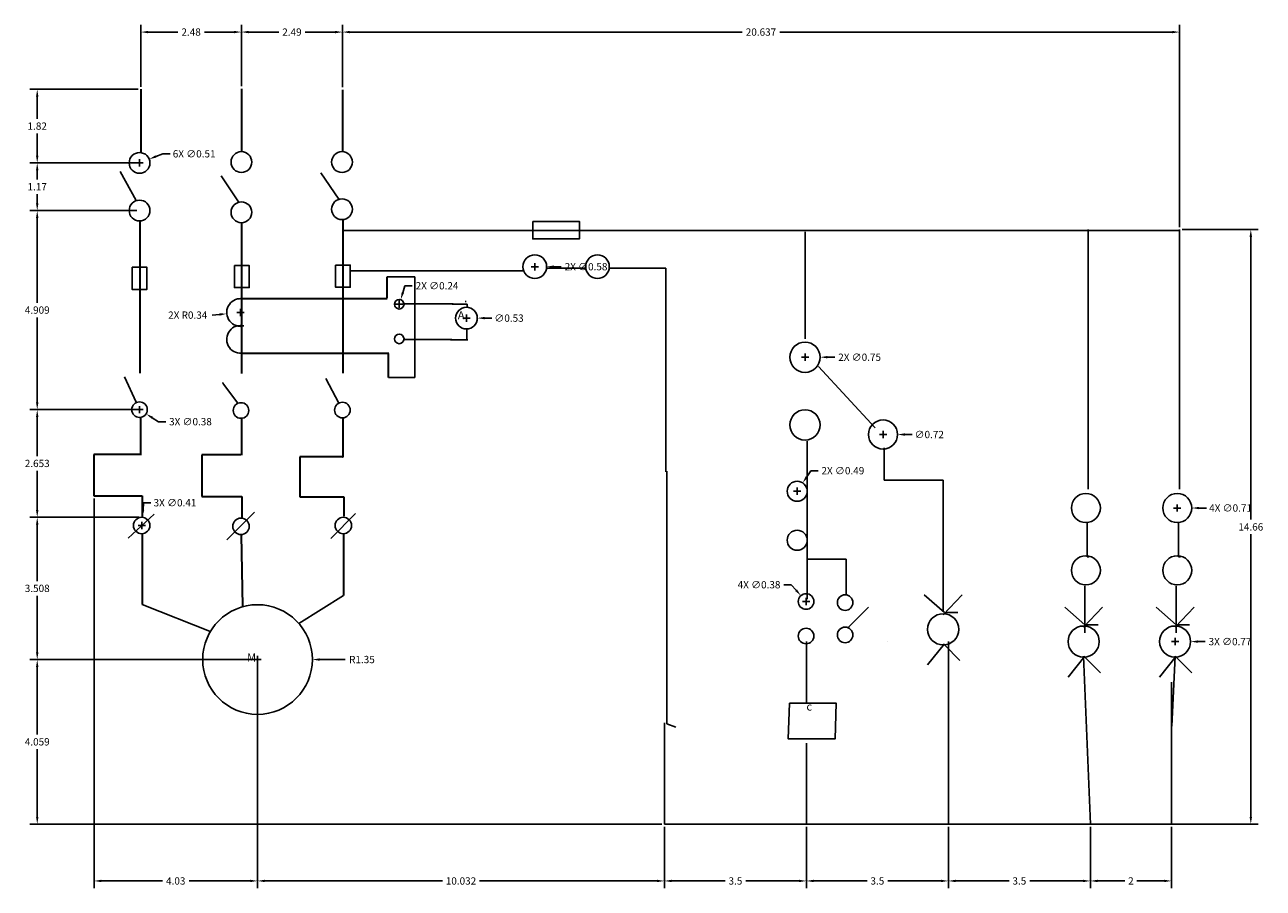
# Model space of a CAD drawing. Units: millimetres. Extents: x 17.2 to 47.7, y -5.7 to 15.6.
import ezdxf

# ---------------------------------------------------------------- set-up
doc = ezdxf.new("R2010")
doc.units = ezdxf.units.MM
doc.header["$MEASUREMENT"] = 0
for name, color, linetype, lineweight in [('A-ANNO-DIMS', 2, 'Continuous', 18), ('E-ANNO-TEXT', 7, 'Continuous', 18), ('E-CTRL-WIRE', 5, 'Continuous', 25), ('E-DEVC-SYMB', 3, 'Continuous', 25), ('E-POWR-WIRE', 1, 'Continuous', 35)]:
    doc.layers.add(name, color=color, linetype=linetype, lineweight=lineweight)
doc.styles.get("Standard").update_dxf_attribs({"font": 'arial.ttf'})
doc.dimstyles.get("Standard").update_dxf_attribs({"dimtxt": 0.18, "dimasz": 0.18, "dimexe": 0.18, "dimexo": 0.0625, "dimgap": 0.09, "dimtad": 0, "dimtih": 1, "dimtoh": 1, "dimdec": 4, "dimzin": 0, "dimdsep": 46, "dimtxsty": 'Standard', "dimcen": 0.09, "dimadec": 0, "dimazin": 0, "dimtfac": 1, "dimtdec": 4, "dimtofl": 0, "dimtmove": 0, "dimatfit": 3, "dimfxl": 1, "dimtolj": 1, "dimtzin": 0, "dimarcsym": 0})

# ---------------------------------------------------------------- blocks, each defined once
blk = doc.blocks.new('*D2')
at = {"layer": 'A-ANNO-DIMS', "color": 0, "lineweight": -2, "transparency": 16777216}
for p, q in [((20.016, 14.072), (20.016, 15.6)), ((22.496, 14.082), (22.496, 15.6)), ((20.196, 15.42), (20.931, 15.42)), ((22.316, 15.42), (21.582, 15.42))]:
    blk.add_line(p, q, dxfattribs=at)
at = {"layer": 'A-ANNO-DIMS', "color": 0, "transparency": 16777216}
for points in [[(20.196, 15.45), (20.196, 15.39), (20.016, 15.42)], [(22.316, 15.45), (22.316, 15.39), (22.496, 15.42)]]:
    blk.add_solid(points, dxfattribs=at)
at = {"layer": 'Defpoints', "color": 0, "transparency": 16777216}
for p in [(22.496, 15.42), (20.016, 14.009), (22.496, 14.02)]:
    blk.add_point(p, dxfattribs=at)
at = {"layer": 'A-ANNO-DIMS', "color": 0, "transparency": 16777216, "insert": (21.256, 15.42), "char_height": 0.18, "attachment_point": 5}
blk.add_mtext('\\A1;2.48', dxfattribs=at)
blk = doc.blocks.new('*D3')
at = {"layer": 'A-ANNO-DIMS', "color": 0, "lineweight": -2, "transparency": 16777216}
for p, q in [((22.496, 14.082), (22.496, 15.6)), ((24.987, 14.061), (24.987, 15.6)), ((22.676, 15.42), (23.416, 15.42)), ((24.807, 15.42), (24.067, 15.42))]:
    blk.add_line(p, q, dxfattribs=at)
at = {"layer": 'A-ANNO-DIMS', "color": 0, "transparency": 16777216}
for points in [[(22.676, 15.45), (22.676, 15.39), (22.496, 15.42)], [(24.807, 15.45), (24.807, 15.39), (24.987, 15.42)]]:
    blk.add_solid(points, dxfattribs=at)
at = {"layer": 'Defpoints', "color": 0, "transparency": 16777216}
for p in [(24.987, 15.42), (22.496, 14.02), (24.987, 13.999)]:
    blk.add_point(p, dxfattribs=at)
at = {"layer": 'A-ANNO-DIMS', "color": 0, "transparency": 16777216, "insert": (23.741, 15.42), "char_height": 0.18, "attachment_point": 5}
blk.add_mtext('\\A1;2.49', dxfattribs=at)
blk = doc.blocks.new('*D4')
at = {"layer": 'A-ANNO-DIMS', "color": 0, "lineweight": -2, "transparency": 16777216}
for p, q in [((24.987, 14.061), (24.987, 15.6)), ((45.623, 10.611), (45.623, 15.6)), ((25.167, 15.42), (34.84, 15.42)), ((45.443, 15.42), (35.77, 15.42))]:
    blk.add_line(p, q, dxfattribs=at)
at = {"layer": 'A-ANNO-DIMS', "color": 0, "transparency": 16777216}
for points in [[(25.167, 15.45), (25.167, 15.39), (24.987, 15.42)], [(45.443, 15.45), (45.443, 15.39), (45.623, 15.42)]]:
    blk.add_solid(points, dxfattribs=at)
at = {"layer": 'Defpoints', "color": 0, "transparency": 16777216}
for p in [(45.623, 15.42), (24.987, 13.999), (45.623, 10.549)]:
    blk.add_point(p, dxfattribs=at)
at = {"layer": 'A-ANNO-DIMS', "color": 0, "transparency": 16777216, "insert": (35.305, 15.42), "char_height": 0.18, "attachment_point": 5}
blk.add_mtext('\\A1;20.637', dxfattribs=at)
blk = doc.blocks.new('*D5')
at = {"layer": 'A-ANNO-DIMS', "color": 0, "lineweight": -2, "transparency": 16777216}
for p, q in [((18.862, 3.921), (18.862, -5.69)), ((22.893, -0.113), (22.893, -5.69)), ((19.042, -5.51), (20.55, -5.51)), ((22.713, -5.51), (21.205, -5.51))]:
    blk.add_line(p, q, dxfattribs=at)
at = {"layer": 'A-ANNO-DIMS', "color": 0, "transparency": 16777216}
for points in [[(19.042, -5.48), (19.042, -5.54), (18.862, -5.51)], [(22.713, -5.48), (22.713, -5.54), (22.893, -5.51)]]:
    blk.add_solid(points, dxfattribs=at)
at = {"layer": 'Defpoints', "color": 0, "transparency": 16777216}
for p in [(18.862, 3.983), (22.893, -0.051), (22.893, -5.51)]:
    blk.add_point(p, dxfattribs=at)
at = {"layer": 'A-ANNO-DIMS', "color": 0, "transparency": 16777216, "insert": (20.877, -5.51), "char_height": 0.18, "attachment_point": 5}
blk.add_mtext('\\A1;4.03', dxfattribs=at)
blk = doc.blocks.new('*D6')
at = {"layer": 'A-ANNO-DIMS', "color": 0, "lineweight": -2, "transparency": 16777216}
for p, q in [((22.893, -0.113), (22.893, -5.69)), ((32.925, -4.172), (32.925, -5.69)), ((23.073, -5.51), (27.455, -5.51)), ((32.745, -5.51), (28.364, -5.51))]:
    blk.add_line(p, q, dxfattribs=at)
at = {"layer": 'A-ANNO-DIMS', "color": 0, "transparency": 16777216}
for points in [[(23.073, -5.48), (23.073, -5.54), (22.893, -5.51)], [(32.745, -5.48), (32.745, -5.54), (32.925, -5.51)]]:
    blk.add_solid(points, dxfattribs=at)
at = {"layer": 'Defpoints', "color": 0, "transparency": 16777216}
for p in [(22.893, -0.051), (32.925, -4.11), (32.925, -5.51)]:
    blk.add_point(p, dxfattribs=at)
at = {"layer": 'A-ANNO-DIMS', "color": 0, "transparency": 16777216, "insert": (27.909, -5.51), "char_height": 0.18, "attachment_point": 5}
blk.add_mtext('\\A1;10.032', dxfattribs=at)
blk = doc.blocks.new('*D7')
at = {"layer": 'A-ANNO-DIMS', "color": 0, "lineweight": -2, "transparency": 16777216}
for p, q in [((32.925, -4.172), (32.925, -5.69)), ((36.425, -4.172), (36.425, -5.69)), ((33.105, -5.51), (34.421, -5.51)), ((36.245, -5.51), (34.93, -5.51))]:
    blk.add_line(p, q, dxfattribs=at)
at = {"layer": 'A-ANNO-DIMS', "color": 0, "transparency": 16777216}
for points in [[(33.105, -5.48), (33.105, -5.54), (32.925, -5.51)], [(36.245, -5.48), (36.245, -5.54), (36.425, -5.51)]]:
    blk.add_solid(points, dxfattribs=at)
at = {"layer": 'Defpoints', "color": 0, "transparency": 16777216}
for p in [(32.925, -4.11), (36.425, -4.11), (36.425, -5.51)]:
    blk.add_point(p, dxfattribs=at)
at = {"layer": 'A-ANNO-DIMS', "color": 0, "transparency": 16777216, "insert": (34.675, -5.51), "char_height": 0.18, "attachment_point": 5}
blk.add_mtext('\\A1;3.5', dxfattribs=at)
blk = doc.blocks.new('*D8')
at = {"layer": 'A-ANNO-DIMS', "color": 0, "lineweight": -2, "transparency": 16777216}
for p, q in [((36.425, -4.172), (36.425, -5.69)), ((39.925, -4.172), (39.925, -5.69)), ((36.605, -5.51), (37.921, -5.51)), ((39.745, -5.51), (38.43, -5.51))]:
    blk.add_line(p, q, dxfattribs=at)
at = {"layer": 'A-ANNO-DIMS', "color": 0, "transparency": 16777216}
for points in [[(36.605, -5.48), (36.605, -5.54), (36.425, -5.51)], [(39.745, -5.48), (39.745, -5.54), (39.925, -5.51)]]:
    blk.add_solid(points, dxfattribs=at)
at = {"layer": 'Defpoints', "color": 0, "transparency": 16777216}
for p in [(36.425, -4.11), (39.925, -4.11), (39.925, -5.51)]:
    blk.add_point(p, dxfattribs=at)
at = {"layer": 'A-ANNO-DIMS', "color": 0, "transparency": 16777216, "insert": (38.175, -5.51), "char_height": 0.18, "attachment_point": 5}
blk.add_mtext('\\A1;3.5', dxfattribs=at)
blk = doc.blocks.new('*D9')
at = {"layer": 'A-ANNO-DIMS', "color": 0, "lineweight": -2, "transparency": 16777216}
for p, q in [((39.925, -4.172), (39.925, -5.69)), ((43.425, -4.172), (43.425, -5.69)), ((40.105, -5.51), (41.421, -5.51)), ((43.245, -5.51), (41.93, -5.51))]:
    blk.add_line(p, q, dxfattribs=at)
at = {"layer": 'A-ANNO-DIMS', "color": 0, "transparency": 16777216}
for points in [[(40.105, -5.48), (40.105, -5.54), (39.925, -5.51)], [(43.245, -5.48), (43.245, -5.54), (43.425, -5.51)]]:
    blk.add_solid(points, dxfattribs=at)
at = {"layer": 'Defpoints', "color": 0, "transparency": 16777216}
for p in [(39.925, -4.11), (43.425, -4.11), (43.425, -5.51)]:
    blk.add_point(p, dxfattribs=at)
at = {"layer": 'A-ANNO-DIMS', "color": 0, "transparency": 16777216, "insert": (41.675, -5.51), "char_height": 0.18, "attachment_point": 5}
blk.add_mtext('\\A1;3.5', dxfattribs=at)
blk = doc.blocks.new('*D10')
at = {"layer": 'A-ANNO-DIMS', "color": 0, "lineweight": -2, "transparency": 16777216}
for p, q in [((43.425, -4.172), (43.425, -5.69)), ((45.425, -4.172), (45.425, -5.69)), ((43.605, -5.51), (44.276, -5.51)), ((45.245, -5.51), (44.575, -5.51))]:
    blk.add_line(p, q, dxfattribs=at)
at = {"layer": 'A-ANNO-DIMS', "color": 0, "transparency": 16777216}
for points in [[(43.605, -5.48), (43.605, -5.54), (43.425, -5.51)], [(45.245, -5.48), (45.245, -5.54), (45.425, -5.51)]]:
    blk.add_solid(points, dxfattribs=at)
at = {"layer": 'Defpoints', "color": 0, "transparency": 16777216}
for p in [(43.425, -4.11), (45.425, -4.11), (45.425, -5.51)]:
    blk.add_point(p, dxfattribs=at)
at = {"layer": 'A-ANNO-DIMS', "color": 0, "transparency": 16777216, "insert": (44.425, -5.51), "char_height": 0.18, "attachment_point": 5}
blk.add_mtext('\\A1;2', dxfattribs=at)
blk = doc.blocks.new('*D11')
at = {"layer": 'A-ANNO-DIMS', "color": 0, "lineweight": -2, "transparency": 16777216}
for p, q in [((45.686, 10.549), (47.561, 10.549)), ((47.381, 10.369), (47.381, 3.401)), ((47.381, -3.93), (47.381, 3.038)), ((45.488, -4.11), (47.561, -4.11))]:
    blk.add_line(p, q, dxfattribs=at)
at = {"layer": 'A-ANNO-DIMS', "color": 0, "transparency": 16777216}
for points in [[(47.351, 10.369), (47.411, 10.369), (47.381, 10.549)], [(47.351, -3.93), (47.411, -3.93), (47.381, -4.11)]]:
    blk.add_solid(points, dxfattribs=at)
at = {"layer": 'Defpoints', "color": 0, "transparency": 16777216}
for p in [(45.623, 10.549), (47.381, 10.549), (45.425, -4.11)]:
    blk.add_point(p, dxfattribs=at)
at = {"layer": 'A-ANNO-DIMS', "color": 0, "transparency": 16777216, "insert": (47.381, 3.219), "char_height": 0.18, "attachment_point": 5}
blk.add_mtext('\\A1;14.66', dxfattribs=at)
blk = doc.blocks.new('*D12')
at = {"layer": 'A-ANNO-DIMS', "color": 0, "lineweight": -2, "transparency": 16777216}
for p, q in [((19.954, 14.009), (17.282, 14.009)), ((17.462, 13.829), (17.462, 13.283)), ((17.462, 12.374), (17.462, 12.92)), ((19.921, 12.194), (17.282, 12.194))]:
    blk.add_line(p, q, dxfattribs=at)
at = {"layer": 'A-ANNO-DIMS', "color": 0, "transparency": 16777216}
for points in [[(17.432, 13.829), (17.492, 13.829), (17.462, 14.009)], [(17.432, 12.374), (17.492, 12.374), (17.462, 12.194)]]:
    blk.add_solid(points, dxfattribs=at)
at = {"layer": 'Defpoints', "color": 0, "transparency": 16777216}
for p in [(20.016, 14.009), (17.462, 12.194), (19.984, 12.194)]:
    blk.add_point(p, dxfattribs=at)
at = {"layer": 'A-ANNO-DIMS', "color": 0, "transparency": 16777216, "insert": (17.462, 13.101), "char_height": 0.18, "attachment_point": 5}
blk.add_mtext('\\A1;1.82', dxfattribs=at)
blk = doc.blocks.new('*D13')
at = {"layer": 'A-ANNO-DIMS', "color": 0, "lineweight": -2, "transparency": 16777216}
for p, q in [((19.921, 12.194), (17.282, 12.194)), ((17.462, 12.014), (17.462, 11.787)), ((17.462, 11.199), (17.462, 11.426)), ((19.921, 11.019), (17.282, 11.019))]:
    blk.add_line(p, q, dxfattribs=at)
at = {"layer": 'A-ANNO-DIMS', "color": 0, "transparency": 16777216}
for points in [[(17.432, 12.014), (17.492, 12.014), (17.462, 12.194)], [(17.432, 11.199), (17.492, 11.199), (17.462, 11.019)]]:
    blk.add_solid(points, dxfattribs=at)
at = {"layer": 'Defpoints', "color": 0, "transparency": 16777216}
for p in [(19.984, 12.194), (17.462, 11.019), (19.984, 11.019)]:
    blk.add_point(p, dxfattribs=at)
at = {"layer": 'A-ANNO-DIMS', "color": 0, "transparency": 16777216, "insert": (17.462, 11.606), "char_height": 0.18, "attachment_point": 5}
blk.add_mtext('\\A1;1.17', dxfattribs=at)
blk = doc.blocks.new('*D14')
at = {"layer": 'A-ANNO-DIMS', "color": 0, "lineweight": -2, "transparency": 16777216}
for p, q in [((19.921, 11.019), (17.282, 11.019)), ((17.462, 10.839), (17.462, 8.746)), ((17.462, 6.29), (17.462, 8.383)), ((19.922, 6.11), (17.282, 6.11))]:
    blk.add_line(p, q, dxfattribs=at)
at = {"layer": 'A-ANNO-DIMS', "color": 0, "transparency": 16777216}
for points in [[(17.432, 10.839), (17.492, 10.839), (17.462, 11.019)], [(17.432, 6.29), (17.492, 6.29), (17.462, 6.11)]]:
    blk.add_solid(points, dxfattribs=at)
at = {"layer": 'Defpoints', "color": 0, "transparency": 16777216}
for p in [(19.984, 11.019), (17.462, 6.11), (19.984, 6.11)]:
    blk.add_point(p, dxfattribs=at)
at = {"layer": 'A-ANNO-DIMS', "color": 0, "transparency": 16777216, "insert": (17.462, 8.565), "char_height": 0.18, "attachment_point": 5}
blk.add_mtext('\\A1;4.909', dxfattribs=at)
blk = doc.blocks.new('*D15')
at = {"layer": 'A-ANNO-DIMS', "color": 0, "lineweight": -2, "transparency": 16777216}
for p, q in [((19.922, 6.11), (17.282, 6.11)), ((17.462, 5.93), (17.462, 4.965)), ((17.462, 3.637), (17.462, 4.602)), ((19.975, 3.457), (17.282, 3.457))]:
    blk.add_line(p, q, dxfattribs=at)
at = {"layer": 'A-ANNO-DIMS', "color": 0, "transparency": 16777216}
for points in [[(17.432, 5.93), (17.492, 5.93), (17.462, 6.11)], [(17.432, 3.637), (17.492, 3.637), (17.462, 3.457)]]:
    blk.add_solid(points, dxfattribs=at)
at = {"layer": 'Defpoints', "color": 0, "transparency": 16777216}
for p in [(19.984, 6.11), (17.462, 3.457), (20.038, 3.457)]:
    blk.add_point(p, dxfattribs=at)
at = {"layer": 'A-ANNO-DIMS', "color": 0, "transparency": 16777216, "insert": (17.462, 4.784), "char_height": 0.18, "attachment_point": 5}
blk.add_mtext('\\A1;2.653', dxfattribs=at)
blk = doc.blocks.new('*D16')
at = {"layer": 'A-ANNO-DIMS', "color": 0, "lineweight": -2, "transparency": 16777216}
for p, q in [((19.975, 3.457), (17.282, 3.457)), ((17.462, 3.277), (17.462, 1.885)), ((17.462, 0.129), (17.462, 1.521)), ((22.831, -0.051), (17.282, -0.051))]:
    blk.add_line(p, q, dxfattribs=at)
at = {"layer": 'A-ANNO-DIMS', "color": 0, "transparency": 16777216}
for points in [[(17.432, 3.277), (17.492, 3.277), (17.462, 3.457)], [(17.432, 0.129), (17.492, 0.129), (17.462, -0.051)]]:
    blk.add_solid(points, dxfattribs=at)
at = {"layer": 'Defpoints', "color": 0, "transparency": 16777216}
for p in [(20.038, 3.457), (17.462, -0.051), (22.893, -0.051)]:
    blk.add_point(p, dxfattribs=at)
at = {"layer": 'A-ANNO-DIMS', "color": 0, "transparency": 16777216, "insert": (17.462, 1.703), "char_height": 0.18, "attachment_point": 5}
blk.add_mtext('\\A1;3.508', dxfattribs=at)
blk = doc.blocks.new('*D17')
at = {"layer": 'A-ANNO-DIMS', "color": 0, "lineweight": -2, "transparency": 16777216}
for p, q in [((22.831, -0.051), (17.282, -0.051)), ((17.462, -0.231), (17.462, -1.898)), ((17.462, -3.93), (17.462, -2.262)), ((32.863, -4.11), (17.282, -4.11))]:
    blk.add_line(p, q, dxfattribs=at)
at = {"layer": 'A-ANNO-DIMS', "color": 0, "transparency": 16777216}
for points in [[(17.432, -0.231), (17.492, -0.231), (17.462, -0.051)], [(17.432, -3.93), (17.492, -3.93), (17.462, -4.11)]]:
    blk.add_solid(points, dxfattribs=at)
at = {"layer": 'Defpoints', "color": 0, "transparency": 16777216}
for p in [(22.893, -0.051), (17.462, -4.11), (32.925, -4.11)]:
    blk.add_point(p, dxfattribs=at)
at = {"layer": 'A-ANNO-DIMS', "color": 0, "transparency": 16777216, "insert": (17.462, -2.08), "char_height": 0.18, "attachment_point": 5}
blk.add_mtext('\\A1;4.059', dxfattribs=at)
blk = doc.blocks.new('*D18')
at = {"layer": 'A-ANNO-DIMS', "color": 0, "lineweight": -2, "transparency": 16777216}
for p, q in [((22.893, -0.141), (22.893, 0.039)), ((22.803, -0.051), (22.983, -0.051)), ((25.056, -0.051), (24.425, -0.051))]:
    blk.add_line(p, q, dxfattribs=at)
at = {"layer": 'A-ANNO-DIMS', "color": 0, "transparency": 16777216}
blk.add_solid([(24.425, -0.021), (24.425, -0.081), (24.245, -0.051)], dxfattribs=at)
at = {"layer": 'Defpoints', "color": 0, "transparency": 16777216}
for p in [(22.893, -0.051), (24.245, -0.051)]:
    blk.add_point(p, dxfattribs=at)
at = {"layer": 'A-ANNO-DIMS', "color": 0, "transparency": 16777216, "insert": (25.467, -0.051), "char_height": 0.18, "attachment_point": 5}
blk.add_mtext('\\A1;R1.35', dxfattribs=at)
blk = doc.blocks.new('*D19')
at = {"layer": 'A-ANNO-DIMS', "color": 0, "lineweight": -2, "transparency": 16777216}
for p, q in [((45.423, 0.391), (45.603, 0.391)), ((45.513, 0.301), (45.513, 0.481)), ((46.258, 0.391), (46.078, 0.391))]:
    blk.add_line(p, q, dxfattribs=at)
at = {"layer": 'A-ANNO-DIMS', "color": 0, "transparency": 16777216}
blk.add_solid([(46.078, 0.421), (46.078, 0.361), (45.898, 0.391)], dxfattribs=at)
at = {"layer": 'Defpoints', "color": 0, "transparency": 16777216}
for p in [(45.129, 0.392), (45.898, 0.391)]:
    blk.add_point(p, dxfattribs=at)
at = {"layer": 'A-ANNO-DIMS', "color": 0, "transparency": 16777216, "insert": (46.868, 0.391), "char_height": 0.18, "attachment_point": 5}
blk.add_mtext('\\A1;3X ∅0.77', dxfattribs=at)
blk = doc.blocks.new('*D20')
at = {"layer": 'A-ANNO-DIMS', "color": 0, "lineweight": -2, "transparency": 16777216}
for p, q in [((36.301, 7.403), (36.481, 7.403)), ((36.391, 7.313), (36.391, 7.493)), ((37.124, 7.403), (36.944, 7.403))]:
    blk.add_line(p, q, dxfattribs=at)
at = {"layer": 'A-ANNO-DIMS', "color": 0, "transparency": 16777216}
blk.add_solid([(36.944, 7.433), (36.944, 7.373), (36.764, 7.403)], dxfattribs=at)
at = {"layer": 'Defpoints', "color": 0, "transparency": 16777216}
for p in [(36.017, 7.402), (36.764, 7.403)]:
    blk.add_point(p, dxfattribs=at)
at = {"layer": 'A-ANNO-DIMS', "color": 0, "transparency": 16777216, "insert": (37.737, 7.403), "char_height": 0.18, "attachment_point": 5}
blk.add_mtext('\\A1;2X ∅0.75', dxfattribs=at)
blk = doc.blocks.new('*D21')
at = {"layer": 'A-ANNO-DIMS', "color": 0, "lineweight": -2, "transparency": 16777216}
for p, q in [((38.224, 5.497), (38.404, 5.497)), ((38.314, 5.407), (38.314, 5.587)), ((39.032, 5.497), (38.852, 5.497))]:
    blk.add_line(p, q, dxfattribs=at)
at = {"layer": 'A-ANNO-DIMS', "color": 0, "transparency": 16777216}
blk.add_solid([(38.852, 5.527), (38.852, 5.467), (38.672, 5.497)], dxfattribs=at)
at = {"layer": 'Defpoints', "color": 0, "transparency": 16777216}
for p in [(37.956, 5.498), (38.672, 5.497)]:
    blk.add_point(p, dxfattribs=at)
at = {"layer": 'A-ANNO-DIMS', "color": 0, "transparency": 16777216, "insert": (39.453, 5.497), "char_height": 0.18, "attachment_point": 5}
blk.add_mtext('\\A1;∅0.72', dxfattribs=at)
blk = doc.blocks.new('*D22')
at = {"layer": 'A-ANNO-DIMS', "color": 0, "lineweight": -2, "transparency": 16777216}
for p, q in [((45.478, 3.685), (45.658, 3.685)), ((45.568, 3.595), (45.568, 3.775)), ((46.286, 3.685), (46.106, 3.685))]:
    blk.add_line(p, q, dxfattribs=at)
at = {"layer": 'A-ANNO-DIMS', "color": 0, "transparency": 16777216}
blk.add_solid([(46.106, 3.715), (46.106, 3.655), (45.926, 3.685)], dxfattribs=at)
at = {"layer": 'Defpoints', "color": 0, "transparency": 16777216}
for p in [(45.211, 3.686), (45.926, 3.685)]:
    blk.add_point(p, dxfattribs=at)
at = {"layer": 'A-ANNO-DIMS', "color": 0, "transparency": 16777216, "insert": (46.882, 3.685), "char_height": 0.18, "attachment_point": 5}
blk.add_mtext('\\A1;4X ∅0.71', dxfattribs=at)
blk = doc.blocks.new('*D23')
at = {"layer": 'A-ANNO-DIMS', "color": 0, "lineweight": -2, "transparency": 16777216}
for p, q in [((22.475, 8.416), (22.475, 8.596)), ((21.776, 8.441), (21.955, 8.457)), ((22.385, 8.506), (22.565, 8.506))]:
    blk.add_line(p, q, dxfattribs=at)
at = {"layer": 'A-ANNO-DIMS', "color": 0, "transparency": 16777216}
blk.add_solid([(21.953, 8.487), (21.958, 8.427), (22.135, 8.474)], dxfattribs=at)
at = {"layer": 'Defpoints', "color": 0, "transparency": 16777216}
for p in [(22.135, 8.474), (22.475, 8.506)]:
    blk.add_point(p, dxfattribs=at)
at = {"layer": 'A-ANNO-DIMS', "color": 0, "transparency": 16777216, "insert": (21.172, 8.441), "char_height": 0.18, "attachment_point": 5}
blk.add_mtext('\\A1;2X R0.34', dxfattribs=at)
blk = doc.blocks.new('*D24')
at = {"layer": 'A-ANNO-DIMS', "color": 0, "lineweight": -2, "transparency": 16777216}
for p, q in [((29.639, 9.635), (29.819, 9.635)), ((29.729, 9.545), (29.729, 9.725)), ((30.38, 9.635), (30.2, 9.635))]:
    blk.add_line(p, q, dxfattribs=at)
at = {"layer": 'A-ANNO-DIMS', "color": 0, "transparency": 16777216}
blk.add_solid([(30.2, 9.665), (30.2, 9.605), (30.02, 9.635)], dxfattribs=at)
at = {"layer": 'Defpoints', "color": 0, "transparency": 16777216}
for p in [(29.437, 9.635), (30.02, 9.635)]:
    blk.add_point(p, dxfattribs=at)
at = {"layer": 'A-ANNO-DIMS', "color": 0, "transparency": 16777216, "insert": (30.992, 9.635), "char_height": 0.18, "attachment_point": 5}
blk.add_mtext('\\A1;2X ∅0.58', dxfattribs=at)
blk = doc.blocks.new('*D25')
at = {"layer": 'A-ANNO-DIMS', "color": 0, "lineweight": -2, "transparency": 16777216}
for p, q in [((27.954, 8.367), (28.134, 8.367)), ((28.044, 8.277), (28.044, 8.457)), ((28.671, 8.367), (28.491, 8.367))]:
    blk.add_line(p, q, dxfattribs=at)
at = {"layer": 'A-ANNO-DIMS', "color": 0, "transparency": 16777216}
blk.add_solid([(28.491, 8.397), (28.491, 8.337), (28.311, 8.367)], dxfattribs=at)
at = {"layer": 'Defpoints', "color": 0, "transparency": 16777216}
for p in [(27.777, 8.367), (28.311, 8.367)]:
    blk.add_point(p, dxfattribs=at)
at = {"layer": 'A-ANNO-DIMS', "color": 0, "transparency": 16777216, "insert": (29.093, 8.367), "char_height": 0.18, "attachment_point": 5}
blk.add_mtext('\\A1;∅0.53', dxfattribs=at)
blk = doc.blocks.new('*D26')
at = {"layer": 'A-ANNO-DIMS', "color": 0, "lineweight": -2, "transparency": 16777216}
for p, q in [((26.528, 9.165), (26.475, 8.993)), ((26.708, 9.165), (26.528, 9.165)), ((26.297, 8.709), (26.477, 8.709)), ((26.387, 8.619), (26.387, 8.799))]:
    blk.add_line(p, q, dxfattribs=at)
at = {"layer": 'A-ANNO-DIMS', "color": 0, "transparency": 16777216}
blk.add_solid([(26.446, 9.002), (26.503, 8.984), (26.422, 8.821)], dxfattribs=at)
at = {"layer": 'Defpoints', "color": 0, "transparency": 16777216}
for p in [(26.353, 8.596), (26.422, 8.821)]:
    blk.add_point(p, dxfattribs=at)
at = {"layer": 'A-ANNO-DIMS', "color": 0, "transparency": 16777216, "insert": (27.319, 9.165), "char_height": 0.18, "attachment_point": 5}
blk.add_mtext('\\A1;2X ∅0.24', dxfattribs=at)
blk = doc.blocks.new('*D27')
at = {"layer": 'A-ANNO-DIMS', "color": 0, "lineweight": -2, "transparency": 16777216}
for p, q in [((19.894, 6.11), (20.074, 6.11)), ((19.984, 6.02), (19.984, 6.2)), ((20.45, 5.813), (20.298, 5.91)), ((20.63, 5.813), (20.45, 5.813))]:
    blk.add_line(p, q, dxfattribs=at)
at = {"layer": 'A-ANNO-DIMS', "color": 0, "transparency": 16777216}
blk.add_solid([(20.314, 5.935), (20.282, 5.885), (20.146, 6.007)], dxfattribs=at)
at = {"layer": 'Defpoints', "color": 0, "transparency": 16777216}
for p in [(19.822, 6.214), (20.146, 6.007)]:
    blk.add_point(p, dxfattribs=at)
at = {"layer": 'A-ANNO-DIMS', "color": 0, "transparency": 16777216, "insert": (21.24, 5.813), "char_height": 0.18, "attachment_point": 5}
blk.add_mtext('\\A1;3X ∅0.38', dxfattribs=at)
blk = doc.blocks.new('*D28')
at = {"layer": 'A-ANNO-DIMS', "color": 0, "lineweight": -2, "transparency": 16777216}
for p, q in [((20.086, 3.815), (20.07, 3.636)), ((20.266, 3.815), (20.086, 3.815)), ((19.948, 3.254), (20.128, 3.254)), ((20.038, 3.164), (20.038, 3.344))]:
    blk.add_line(p, q, dxfattribs=at)
at = {"layer": 'A-ANNO-DIMS', "color": 0, "transparency": 16777216}
blk.add_solid([(20.04, 3.638), (20.1, 3.633), (20.055, 3.456)], dxfattribs=at)
at = {"layer": 'Defpoints', "color": 0, "transparency": 16777216}
for p in [(20.055, 3.456), (20.02, 3.052)]:
    blk.add_point(p, dxfattribs=at)
at = {"layer": 'A-ANNO-DIMS', "color": 0, "transparency": 16777216, "insert": (20.858, 3.815), "char_height": 0.18, "attachment_point": 5}
blk.add_mtext('\\A1;3X ∅0.41', dxfattribs=at)
blk = doc.blocks.new('*D29')
at = {"layer": 'A-ANNO-DIMS', "color": 0, "lineweight": -2, "transparency": 16777216}
for p, q in [((36.532, 4.605), (36.433, 4.454)), ((36.712, 4.605), (36.532, 4.605)), ((36.108, 4.097), (36.288, 4.097)), ((36.198, 4.007), (36.198, 4.187))]:
    blk.add_line(p, q, dxfattribs=at)
at = {"layer": 'A-ANNO-DIMS', "color": 0, "transparency": 16777216}
blk.add_solid([(36.408, 4.471), (36.458, 4.438), (36.334, 4.304)], dxfattribs=at)
at = {"layer": 'Defpoints', "color": 0, "transparency": 16777216}
for p in [(36.334, 4.304), (36.062, 3.891)]:
    blk.add_point(p, dxfattribs=at)
at = {"layer": 'A-ANNO-DIMS', "color": 0, "transparency": 16777216, "insert": (37.324, 4.605), "char_height": 0.18, "attachment_point": 5}
blk.add_mtext('\\A1;2X ∅0.49', dxfattribs=at)
blk = doc.blocks.new('*D30')
at = {"layer": 'A-ANNO-DIMS', "color": 0, "lineweight": -2, "transparency": 16777216}
for p, q in [((35.872, 1.793), (36.052, 1.793)), ((36.052, 1.793), (36.171, 1.658)), ((36.328, 1.38), (36.508, 1.38)), ((36.418, 1.29), (36.418, 1.47))]:
    blk.add_line(p, q, dxfattribs=at)
at = {"layer": 'A-ANNO-DIMS', "color": 0, "transparency": 16777216}
blk.add_solid([(36.193, 1.678), (36.149, 1.638), (36.291, 1.523)], dxfattribs=at)
at = {"layer": 'Defpoints', "color": 0, "transparency": 16777216}
for p in [(36.291, 1.523), (36.546, 1.236)]:
    blk.add_point(p, dxfattribs=at)
at = {"layer": 'A-ANNO-DIMS', "color": 0, "transparency": 16777216, "insert": (35.257, 1.793), "char_height": 0.18, "attachment_point": 5}
blk.add_mtext('\\A1;4X ∅0.38', dxfattribs=at)
blk = doc.blocks.new('*D31')
at = {"layer": 'A-ANNO-DIMS', "color": 0, "lineweight": -2, "transparency": 16777216}
for p, q in [((19.984, 12.104), (19.984, 12.284)), ((20.558, 12.418), (20.39, 12.353)), ((20.738, 12.418), (20.558, 12.418)), ((19.894, 12.194), (20.074, 12.194))]:
    blk.add_line(p, q, dxfattribs=at)
at = {"layer": 'A-ANNO-DIMS', "color": 0, "transparency": 16777216}
blk.add_solid([(20.379, 12.381), (20.401, 12.325), (20.223, 12.287)], dxfattribs=at)
at = {"layer": 'Defpoints', "color": 0, "transparency": 16777216}
for p in [(20.223, 12.287), (19.745, 12.1)]:
    blk.add_point(p, dxfattribs=at)
at = {"layer": 'A-ANNO-DIMS', "color": 0, "transparency": 16777216, "insert": (21.331, 12.418), "char_height": 0.18, "attachment_point": 5}
blk.add_mtext('\\A1;6X ∅0.51', dxfattribs=at)

msp = doc.modelspace()

# ---------------------------------------------------------------- linework, layer by layer
at = {"layer": 'E-CTRL-WIRE'}
for p, q in [((25.0057, 10.5274), (45.5958, 10.5274)), ((36.3906, 10.4938), (36.3906, 7.8583)), ((43.3701, 10.5487), (43.3701, 4.1523)), ((45.6233, 10.5487), (45.6233, 4.1523)), ((25.1775, 9.5323), (29.4366, 9.5323)), ((30.0377, 9.6009), (30.9994, 9.6009)), ((31.549, 9.6009), (32.9572, 9.6009)), ((32.9572, 9.6009), (32.9572, 4.5737)), ((26.0879, 9.3814), (26.7721, 9.3814)), ((26.7721, 9.3814), (26.7721, 6.9037)), ((26.5048, 8.7193), (27.7128, 8.7193)), ((28.0656, 8.7086), (27.6914, 8.7086)), ((28.0549, 8.0999), (28.0549, 7.8329)), ((26.5048, 7.8435), (27.1569, 7.8435)), ((28.0762, 7.8329), (27.6486, 7.8329)), ((36.7204, 7.172), (38.1217, 5.6622)), ((26.7721, 6.9037), (26.12, 6.9037)), ((36.4456, 5.3327), (36.4456, 1.4345)), ((38.3416, 5.168), (38.3416, 4.3719)), ((32.9833, -1.2009), (32.9833, 4.5915)), ((38.3416, 4.3719), (39.7979, 4.3719)), ((39.7979, 4.3719), (39.7979, 1.16)), ((43.3426, 3.3287), (43.3426, 2.4777)), ((45.5958, 3.3287), (45.5958, 2.4777)), ((36.4456, 2.4228), (37.4073, 2.4228)), ((37.4073, 2.4228), (37.4073, 1.5443)), ((43.2876, 1.7639), (43.2876, 0.6109)), ((45.5409, 1.7639), (45.5409, 0.6109)), ((39.8529, 1.1051), (40.1551, 1.1051)), ((43.3151, 0.8031), (43.6174, 0.8031)), ((45.5683, 0.8031), (45.8706, 0.8031)), ((36.4255, 0.3901), (36.4255, -0.1099)), ((39.9255, -4.1099), (39.9255, 0.3901)), ((43.2602, 0.0344), (43.4255, -4.1099)), ((36.4255, -0.1099), (36.4255, -1.1099)), ((45.4255, -0.6099), (45.4255, -4.1099)), ((32.9833, -1.6401), (32.9833, -1.0362)), ((32.9255, -1.6099), (32.9255, -4.1099)), ((36.4255, -4.1099), (36.4255, -2.1099)), ((32.9255, -4.1099), (33.4255, -4.1099)), ((45.6905, -4.1099), (33.1604, -4.1099))]:
    msp.add_line(p, q, dxfattribs=at)
at = {"layer": 'E-DEVC-SYMB'}
for p, q in [((19.8985, 11.2646), (19.5029, 11.9801)), ((24.9013, 11.2966), (24.4523, 11.9481)), ((22.4212, 11.2325), (21.9936, 11.8733)), ((31.6005, 9.6009), (31.549, 9.6009)), ((28.0335, 8.7727), (28.0121, 8.7727)), ((28.0656, 8.6338), (28.0656, 8.7086)), ((27.1569, 7.8435), (27.3066, 7.8435)), ((27.3066, 7.8435), (27.3921, 7.8435)), ((27.3921, 7.8435), (27.4455, 7.8435)), ((27.4455, 7.8435), (27.5952, 7.8435)), ((27.5952, 7.8435), (27.6807, 7.8435)), ((27.6807, 7.8435), (27.6807, 7.8435)), ((28.0549, 7.8329), (28.0762, 7.8329)), ((19.8986, 6.2917), (19.61, 6.9218)), ((19.61, 6.9218), (19.61, 6.9218)), ((22.0365, 6.7723), (22.0365, 6.783)), ((22.0579, 6.7402), (22.0365, 6.7723)), ((22.4107, 6.2703), (22.0579, 6.7402)), ((24.9014, 6.2703), (24.5807, 6.8791)), ((24.9976, 4.9354), (24.9869, 4.9354)), ((43.3701, 4.1523), (43.3701, 4.2346)), ((45.6233, 4.1523), (45.6233, 4.2346)), ((20.3475, 3.5317), (19.7061, 2.9443)), ((22.8168, 3.5851), (22.1327, 2.9016)), ((25.3076, 3.553), (24.6982, 2.9336)), ((43.3426, 2.4777), (43.3976, 2.4777)), ((45.5958, 2.4777), (45.6508, 2.4777)), ((25.0097, 1.5297), (23.9087, 0.8356)), ((39.8254, 1.1051), (39.3308, 1.5443)), ((39.7979, 1.0502), (40.265, 1.5443)), ((20.0497, 1.3055), (21.7493, 0.6326)), ((37.4623, 0.7482), (37.9569, 1.2423)), ((43.2876, 0.8031), (42.793, 1.2423)), ((43.2602, 0.7482), (43.7273, 1.2423)), ((45.5409, 0.8031), (45.0462, 1.2423)), ((45.5134, 0.7482), (45.9805, 1.2423)), ((38.4255, 0.3901), (38.4255, 0.3901)), ((39.8254, 0.3364), (39.4132, -0.1852)), ((39.8254, 0.309), (40.2101, -0.0754)), ((43.2876, 0.0344), (42.8755, -0.4871)), ((43.2876, 0.007), (43.6723, -0.3773)), ((45.5409, 0.0344), (45.1287, -0.4871)), ((45.5134, 0.0344), (45.4309, -1.695)), ((45.5409, 0.007), (45.9255, -0.3773)), ((33.2032, -1.7225), (32.9833, -1.6401))]:
    msp.add_line(p, q, dxfattribs=at)
for points in [[(29.677, 10.7505), (30.8277, 10.7505), (30.8277, 10.3215), (29.677, 10.3215)], [(19.8022, 9.6199), (20.1657, 9.6199), (20.1657, 9.0752), (19.8022, 9.0752)], [(22.325, 9.6626), (22.6885, 9.6626), (22.6885, 9.118), (22.325, 9.118)], [(24.8157, 9.6733), (25.1792, 9.6733), (25.1792, 9.1286), (24.8157, 9.1286)], [(36.0059, -1.1303), (37.16, -1.1303), (37.1325, -2.0087), (35.9785, -2.0087)]]:
    msp.add_lwpolyline(points, close=True, dxfattribs=at)
for centre, radius in [((19.984, 12.1937), 0.2563), ((22.4958, 12.2151), 0.2563), ((24.9758, 12.2151), 0.2563), ((24.9758, 11.051), 0.2563), ((19.984, 11.019), 0.2563), ((22.4958, 10.9762), 0.2563), ((29.7285, 9.6352), 0.2917), ((31.2742, 9.6352), 0.2917), ((26.3873, 8.7086), 0.1176), ((28.0442, 8.3668), 0.2672), ((26.3873, 7.8542), 0.1176), ((36.3906, 7.4026), 0.3734), ((19.9841, 6.1101), 0.1924), ((22.4855, 6.0888), 0.1924), ((24.9869, 6.0996), 0.1924), ((36.3906, 5.7336), 0.3734), ((38.3141, 5.4975), 0.3582), ((36.1983, 4.0974), 0.2473), ((43.3151, 3.6853), 0.3572), ((45.5683, 3.6853), 0.3572), ((20.0375, 3.254), 0.2029), ((22.4853, 3.2326), 0.2029), ((25.0081, 3.254), 0.2029), ((36.1983, 2.8895), 0.2473), ((43.3151, 2.1486), 0.3572), ((45.5683, 2.1486), 0.3572), ((36.4181, 1.3796), 0.1922), ((37.3797, 1.3522), 0.1922), ((22.8931, -0.0509), 1.3518), ((39.7979, 0.6933), 0.3843), ((36.4179, 0.5286), 0.1922), ((37.3797, 0.556), 0.1922), ((43.2602, 0.3913), 0.3843), ((45.5134, 0.3913), 0.3843)]:
    msp.add_circle(centre, radius, dxfattribs=at)
for centre, start, end in [((22.4748, 8.5057), 86.43303, 284.36152), ((22.4748, 7.8435), 75.63848, 273.56697)]:
    msp.add_arc(centre, 0.3418, start, end, dxfattribs=at)
at = {"layer": 'E-POWR-WIRE'}
for p, q in [((20.016, 14.0093), (20.016, 12.4607)), ((22.4961, 14.0199), (22.4961, 12.4821)), ((24.9868, 13.9986), (24.9868, 12.4821)), ((19.9947, 10.752), (19.9947, 7.0105)), ((22.4961, 10.7092), (22.4961, 6.9998)), ((24.9975, 10.784), (24.9975, 7.0105)), ((26.0879, 8.8581), (26.0879, 9.3814)), ((22.4748, 8.8474), (26.0879, 8.8474)), ((22.4855, 7.5018), (23.8324, 7.5018)), ((23.8324, 7.5018), (26.1307, 7.5018)), ((26.12, 6.9037), (26.12, 7.4911)), ((20.0055, 5.9179), (20.0055, 4.9888)), ((22.4962, 5.8965), (22.4962, 4.9888)), ((24.9976, 5.9286), (24.9976, 4.9354)), ((19.9947, 5.0084), (18.8616, 5.0084)), ((18.8616, 5.0084), (18.8616, 3.9831)), ((22.4855, 4.9977), (21.5234, 4.9977)), ((21.5234, 4.9977), (21.5234, 3.9724)), ((25.0082, 4.9443), (23.9393, 4.9443)), ((23.9393, 4.9443), (23.9393, 3.9618)), ((18.8616, 3.9831), (20.0482, 3.9831)), ((20.0482, 3.9831), (20.0482, 3.4705)), ((21.5234, 3.9724), (22.5068, 3.9724)), ((22.5068, 3.9724), (22.5068, 3.4598)), ((23.9393, 3.9618), (25.0189, 3.9618)), ((25.0189, 3.9618), (25.0189, 3.4812)), ((20.0497, 3.0569), (20.0497, 1.3055)), ((22.4869, 3.0142), (22.519, 1.2627)), ((25.0097, 3.0356), (25.0097, 1.5297))]:
    msp.add_line(p, q, dxfattribs=at)

# ---------------------------------------------------------------- texts
at = {"layer": 'E-ANNO-TEXT', "char_height": 0.2, "attachment_point": 1}
for s, width, heights, insert in [('A  ', 0.44897, [0.2], (27.8304, 8.5377)), ('M\\P   ', 0.128277, [0], (22.6366, 0.0999))]:
    msp.add_mtext_dynamic_manual_height_columns(s, width=width, gutter_width=1, heights=heights, dxfattribs=dict(at, insert=insert))
at = {"layer": 'E-ANNO-TEXT', "insert": (36.4255, -1.1099), "char_height": 0.2, "attachment_point": 1}
msp.add_mtext('c  ', dxfattribs=at)

# ---------------------------------------------------------------- dimensions: what is measured, and where the dimension line sits
at = {"layer": 'A-ANNO-DIMS'}
for base, p1, p2, override, picture, middle in [((22.4961, 15.42), (20.016, 14.0093), (22.4961, 14.0199), {"dimdec": 2, "dimlfac": 1, "dimrnd": 0, "dimzin": 0, "dimdsep": 46, "dimlunit": 2}, '*D2', (21.2561, 15.42)), ((24.9868, 15.42), (22.4961, 14.0199), (24.9868, 13.9986), {"dimdec": 2, "dimlfac": 1, "dimrnd": 0, "dimzin": 0, "dimdsep": 46, "dimlunit": 2}, '*D3', (23.7414, 15.42)), ((45.62329, 15.41995), (24.98678, 13.99859), (45.62329, 10.54867), {"dimdec": 3, "dimlfac": 1, "dimrnd": 0, "dimzin": 0, "dimdsep": 46, "dimlunit": 2}, '*D4', (35.30503, 15.41995)), ((22.8931, -5.5099), (18.8616, 3.9831), (22.8931, -0.0509), {"dimdec": 2, "dimlfac": 1, "dimrnd": 0, "dimzin": 0, "dimdsep": 46, "dimlunit": 2}, '*D5', (20.8774, -5.5099)), ((32.9255, -5.5099), (22.8931, -0.0509), (32.9255, -4.1099), {"dimdec": 3, "dimlfac": 1, "dimrnd": 0, "dimzin": 0, "dimdsep": 46, "dimlunit": 2}, '*D6', (27.9093, -5.5099)), ((36.4255, -5.5099), (32.9255, -4.1099), (36.4255, -4.1099), {"dimdec": 1, "dimlfac": 1, "dimrnd": 0, "dimzin": 0, "dimdsep": 46, "dimlunit": 2}, '*D7', (34.6755, -5.5099)), ((39.9255, -5.5099), (36.4255, -4.1099), (39.9255, -4.1099), {"dimdec": 1, "dimlfac": 1, "dimrnd": 0, "dimzin": 0, "dimdsep": 46, "dimlunit": 2}, '*D8', (38.1755, -5.5099)), ((43.4255, -5.5099), (39.9255, -4.1099), (43.4255, -4.1099), {"dimdec": 1, "dimlfac": 1, "dimrnd": 0, "dimzin": 0, "dimdsep": 46, "dimlunit": 2}, '*D9', (41.6755, -5.5099)), ((45.4255, -5.5099), (43.4255, -4.1099), (45.4255, -4.1099), {"dimdec": 0, "dimlfac": 1, "dimrnd": 0, "dimzin": 0, "dimdsep": 46, "dimlunit": 2}, '*D10', (44.4255, -5.5099))]:
    dim = msp.add_linear_dim(base=base, p1=p1, p2=p2, dimstyle='Standard', override=override, dxfattribs=at)
    dim.commit()
    dim.dimension.update_dxf_attribs({"geometry": picture, "text_midpoint": middle})
for base, p1, p2, override, picture, middle in [((17.4616, 12.1937), (20.016, 14.0093), (19.984, 12.1937), {"dimdec": 2, "dimlfac": 1, "dimrnd": 0, "dimzin": 0, "dimdsep": 46, "dimlunit": 2}, '*D12', (17.4616, 13.1015)), ((17.4616, 11.019), (19.984, 12.1937), (19.984, 11.019), {"dimdec": 2, "dimlfac": 1, "dimrnd": 0, "dimzin": 0, "dimdsep": 46, "dimlunit": 2}, '*D13', (17.4616, 11.6063)), ((17.4616, 6.1101), (19.984, 11.019), (19.9841, 6.1101), {"dimdec": 3, "dimlfac": 1, "dimrnd": 0, "dimzin": 0, "dimdsep": 46, "dimlunit": 2}, '*D14', (17.4616, 8.5645)), ((47.3805, 10.5487), (45.4255, -4.1099), (45.6233, 10.5487), {"dimdec": 2, "dimlfac": 1, "dimrnd": 0, "dimzin": 0, "dimdsep": 46, "dimlunit": 2}, '*D11', (47.3805, 3.2194)), ((17.4616, 3.4569), (19.9841, 6.1101), (20.0375, 3.4569), {"dimdec": 3, "dimlfac": 1, "dimrnd": 0, "dimzin": 0, "dimdsep": 46, "dimlunit": 2}, '*D15', (17.4616, 4.7835)), ((17.4616, -0.0509), (20.0375, 3.4569), (22.8931, -0.0509), {"dimdec": 3, "dimlfac": 1, "dimrnd": 0, "dimzin": 0, "dimdsep": 46, "dimlunit": 2}, '*D16', (17.4616, 1.703)), ((17.4616, -4.1099), (22.8931, -0.0509), (32.9255, -4.1099), {"dimdec": 3, "dimlfac": 1, "dimrnd": 0, "dimzin": 0, "dimdsep": 46, "dimlunit": 2}, '*D17', (17.4616, -2.0804))]:
    dim = msp.add_linear_dim(base=base, p1=p1, p2=p2, angle=90, dimstyle='Standard', override=override, dxfattribs=at)
    dim.commit()
    dim.dimension.update_dxf_attribs({"geometry": picture, "text_midpoint": middle})
for p1, p2, text, picture, middle in [((19.7453, 12.1002), (20.2226, 12.2872), '6X <>', '*D31', (21.3312, 12.4185)), ((29.4369, 9.6354), (30.0202, 9.635), '2X <>', '*D24', (30.3802, 9.6347)), ((26.3527, 8.5962), (26.4218, 8.821), '2X <>', '*D26', (27.3192, 9.1651)), ((19.8219, 6.2137), (20.1463, 6.0066), '3X <>', '*D27', (21.2402, 5.813)), ((36.0623, 3.8908), (36.3343, 4.3039), '2X <>', '*D29', (37.3243, 4.6046)), ((20.0202, 3.0518), (20.0548, 3.4562), '3X <>', '*D28', (20.8584, 3.8149)), ((45.2111, 3.6855), (45.9255, 3.685), '4X <>', '*D22', (46.2855, 3.6847)), ((36.5457, 1.2359), (36.2905, 1.5233), '4X <>', '*D30', (35.2574, 1.7925))]:
    dim = msp.add_diameter_dim_2p(p1=p1, p2=p2, text=text, dimstyle='Standard', override={"dimdec": 2, "dimlfac": 1, "dimrnd": 0, "dimzin": 0, "dimdsep": 46, "dimlunit": 2}, dxfattribs=at)
    dim.commit()
    dim.dimension.update_dxf_attribs({"geometry": picture, "text_midpoint": middle, "dimtype": 163})
dim = msp.add_radius_dim(center=(22.4748, 8.5057), mpoint=(22.1345, 8.474), text='2X <>', dimstyle='Standard', override={"dimdec": 2, "dimlfac": 1, "dimrnd": 0, "dimzin": 0, "dimdsep": 46, "dimlunit": 2}, dxfattribs=at)
dim.commit()
dim.dimension.update_dxf_attribs({"geometry": '*D23', "text_midpoint": (21.1716, 8.4405)})
for p1, p2, picture, middle in [((27.7769, 8.3667), (28.3114, 8.367), '*D25', (28.6714, 8.3672)), ((37.9559, 5.4979), (38.6723, 5.497), '*D21', (39.0323, 5.4965))]:
    dim = msp.add_diameter_dim_2p(p1=p1, p2=p2, dimstyle='Standard', override={"dimdec": 2, "dimlfac": 1, "dimrnd": 0, "dimzin": 0, "dimdsep": 46, "dimlunit": 2}, dxfattribs=at)
    dim.commit()
    dim.dimension.update_dxf_attribs({"geometry": picture, "text_midpoint": middle})
for p1, p2, text, picture, middle in [((36.0172, 7.4021), (36.764, 7.403), '2X <>', '*D20', (37.124, 7.4034)), ((45.129, 0.3916), (45.8977, 0.391), '3X <>', '*D19', (46.2577, 0.3907))]:
    dim = msp.add_diameter_dim_2p(p1=p1, p2=p2, text=text, dimstyle='Standard', override={"dimdec": 2, "dimlfac": 1, "dimrnd": 0, "dimzin": 0, "dimdsep": 46, "dimlunit": 2}, dxfattribs=at)
    dim.commit()
    dim.dimension.update_dxf_attribs({"geometry": picture, "text_midpoint": middle})
dim = msp.add_radius_dim(center=(22.8931, -0.0509), mpoint=(24.245, -0.051), dimstyle='Standard', override={"dimdec": 2, "dimlfac": 1, "dimrnd": 0, "dimzin": 0, "dimdsep": 46, "dimlunit": 2}, dxfattribs=at)
dim.commit()
dim.dimension.update_dxf_attribs({"geometry": '*D18', "text_midpoint": (25.0561, -0.0511), "dimtype": 164})

doc.saveas('drawing.dxf')
